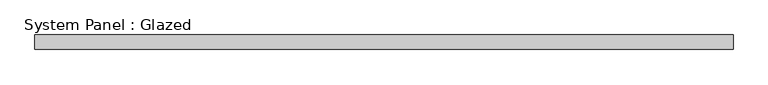
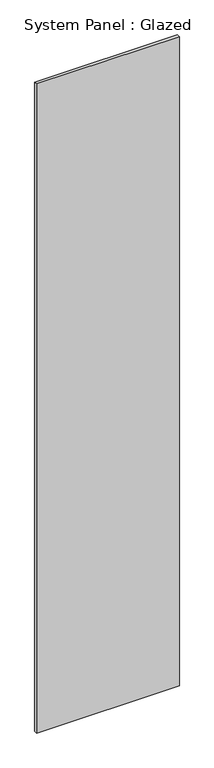
"""IFC4 building model written with IfcOpenShell, lengths in millimetres: plate geometry, System Panel : Glazed."""

from ifc_helpers import new_model, si_unit, origin, origin_with_axes, place, context, project, spatial, polyline, outline, extrude, source, transform, mapped, element, save


def system_panel_glazed_d8816065(model_context):
    return source(origin(), model_context, "Body", "SweptSolid", [
        extrude(outline(polyline([(612.775, 19.05), (-612.775, 19.05), (-612.775, 44.45), (612.775, 44.45), (612.775, 19.05)])), origin_with_axes(), (0.0, 0.0, 1.0), 5884.7116741),
    ])


if __name__ == "__main__":
    model = new_model("IFC4")
    model_context = context("Model", 3, world=origin())
    ifc_project = project(units=[si_unit("LENGTHUNIT", "METRE", prefix="MILLI")], contexts=[model_context])
    site = spatial("IfcSite", under=ifc_project)
    building = spatial("IfcBuilding", under=site)
    placement = place(None, origin())
    system_panel_glazed_shape = system_panel_glazed_d8816065(model_context)
    element("IfcPlate", 1, ObjectType="System Panel : Glazed", at=placement, inside=building, context=model_context, shape_type="MappedRepresentation", body=[
        mapped(system_panel_glazed_shape, transform((0.0, 0.0, 0.0), x_axis=(1.0, 0.0, 0.0), y_axis=(0.0, 1.0, 0.0), z_axis=(0.0, 0.0, 1.0))),
    ])
    save(model, "model.ifc")

# Revit data of these elements
# Type "System Panel : Glazed"
#   Construction Type Id = "GSP4R"
#   Analytic Construction = "1/8 in Pilkington single glazing"
#   Visual Light Transmittance = 0.9
#   Solar Heat Gain Coefficient = 0.86
#   Heat Transfer Coefficient (U) = 1.18115 BTU/(h·ft²·°F)
# Element 1 (IfcPlate, "System Panel : Glazed")
#   Materials on its faces: "Glass"
# Materials
#   "Glass": class "Glass", colour RGB 0 128 192, transparency 0.75, Description = "Soda Lime Glass", Cost = 0
